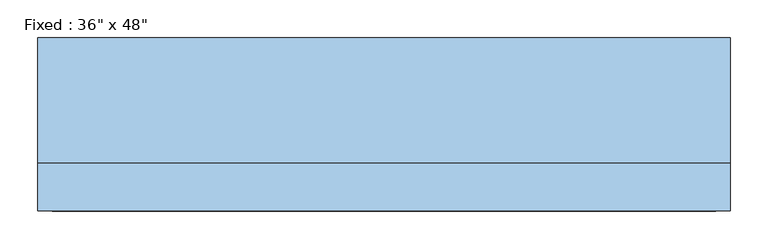
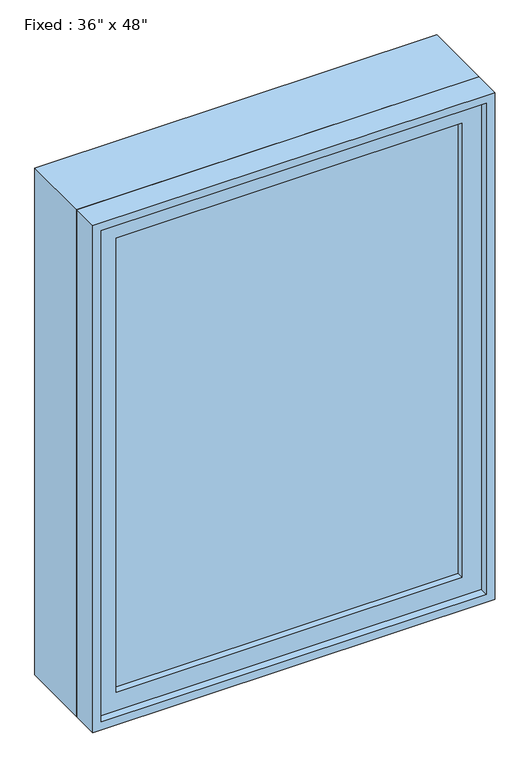
"""IFC4 building model written with IfcOpenShell, lengths in millimetres: window geometry."""

from ifc_helpers import new_model, si_unit, frame, origin, place, context, project, spatial, polyline, outline, extrude, source, transform, mapped, element, save


def window_26734613(model_context):
    return source(origin(), model_context, "Body", "SweptSolid", [
        extrude(outline(polyline([(355.6, -66.675), (355.6, -79.375), (-431.8, -79.375), (-431.8, -66.675), (355.6, -66.675)])), frame((0.0, 0.0, 977.9), z_axis=(0.0, 0.0, 1.0), x_axis=(1.0, 0.0, 0.0)), (0.0, 0.0, 1.0), 1092.2),
        extrude(outline(polyline([(2114.55, -476.25), (933.45, -476.25), (933.45, 400.05), (2114.55, 400.05), (2114.55, -476.25)]), holes=[polyline([(2070.1, -431.8), (2070.1, 355.6), (977.9, 355.6), (977.9, -431.8), (2070.1, -431.8)])]), frame((0.0, -95.25, 0.0), z_axis=(0.0, 1.0, 0.0), x_axis=(0.0, 0.0, 1.0)), (0.0, 0.0, 1.0), 44.45),
        extrude(outline(polyline([(2133.6, -495.3), (914.4, -495.3), (914.4, 419.1), (2133.6, 419.1), (2133.6, -495.3)]), holes=[polyline([(2101.85, -463.55), (2101.85, 387.35), (946.15, 387.35), (946.15, -463.55), (2101.85, -463.55)])]), frame((0.0, -50.8, 0.0), z_axis=(0.0, 1.0, 0.0), x_axis=(0.0, 0.0, 1.0)), (0.0, 0.0, 1.0), 165.1),
        extrude(outline(polyline([(2133.6, 419.1), (2133.6, -495.3), (914.4, -495.3), (914.4, 419.1), (2133.6, 419.1)]), holes=[polyline([(2114.55, 400.05), (933.45, 400.05), (933.45, -476.25), (2114.55, -476.25), (2114.55, 400.05)])]), frame((0.0, -114.3, 0.0), z_axis=(0.0, 1.0, 0.0), x_axis=(0.0, 0.0, 1.0)), (0.0, 0.0, 1.0), 63.5),
    ])


if __name__ == "__main__":
    model = new_model("IFC4")
    model_context = context("Model", 3, world=origin())
    ifc_project = project(units=[si_unit("LENGTHUNIT", "METRE", prefix="MILLI")], contexts=[model_context])
    site = spatial("IfcSite", under=ifc_project)
    building = spatial("IfcBuilding", under=site)
    placement = place(None, origin())
    window_shape = window_26734613(model_context)
    element("IfcWindow", 1, ObjectType="Fixed : 36\" x 48\"", at=placement, inside=building, context=model_context, shape_type="MappedRepresentation", body=[
        mapped(window_shape, transform((0.0, 0.0, 0.0), x_axis=(1.0, 0.0, 0.0), y_axis=(0.0, 1.0, 0.0), z_axis=(0.0, 0.0, 1.0))),
    ])
    save(model, "model.ifc")

# Revit data of these elements
# Type "Fixed : 36\" x 48\""
#   Type Mark = "9"
#   Construction Type Id = "GSP4R"
#   Assembly Code = "B2020100"
#   Analytic Construction = "1/8 in Pilkington single glazing"
#   Visual Light Transmittance = 0.9
#   Solar Heat Gain Coefficient = 0.78
#   Heat Transfer Coefficient (U) = 0.6496 BTU/(h·ft²·°F)
#   Height = 4' - 0"
#   Default Sill Height = 3' - 0"
#   Width = 3' - 0"
#   Window Inset = 0' - 0 3/4"
#   Define Thermal Properties by = 1
#   Wall Closure = 3
#   Glass Pane Material = Glass
#   Sash Material = Sash
# Element 1 (IfcWindow, "Fixed : 36\" x 48\"")
#   Materials on its faces: "Sash", "Glass"
# Materials
#   "Glass": class "Glass", colour RGB 0 128 192, transparency 0.75, Description = "Soda Lime Glass", Cost = 0
#   "Sash": class "Wood", colour RGB 224 178 126, transparency 0
